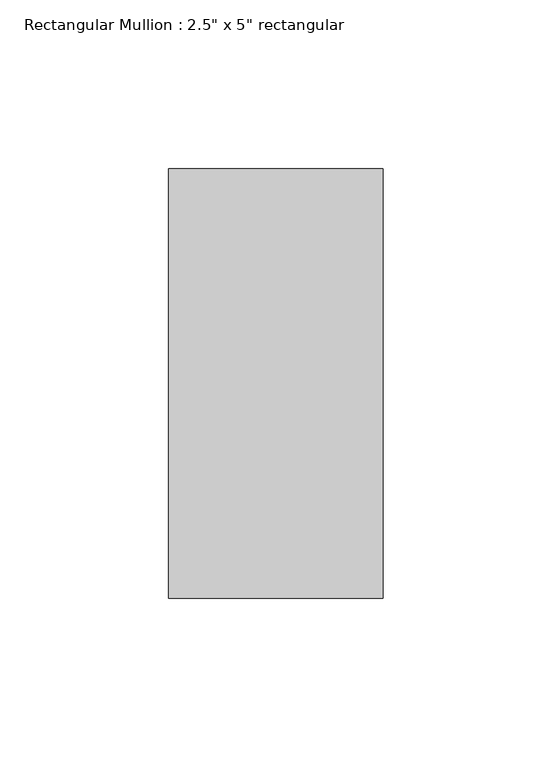
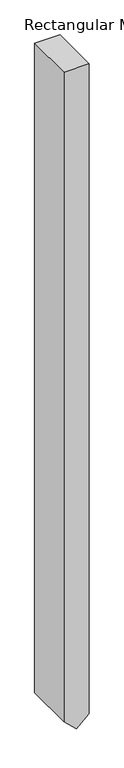
"""IFC4 building model written with IfcOpenShell, lengths in millimetres: member geometry."""

from ifc_helpers import new_model, si_unit, frame, origin, place, context, project, spatial, polyline, outline, extrude, source, transform, mapped, element, save


def member_2e3f679f(model_context):
    return source(origin(), model_context, "Body", "SweptSolid", [
        extrude(outline(polyline([(0.0, 31.75), (0.0, -31.75), (-1725.8468822, -31.75), (-1755.4542362, 0.0), (-1725.8468822, 31.75), (0.0, 31.75)])), frame((0.0, -63.5, 0.0), z_axis=(0.0, 1.0, 0.0), x_axis=(0.0, 0.0, 1.0)), (0.0, 0.0, 1.0), 127.0),
    ])


if __name__ == "__main__":
    model = new_model("IFC4")
    model_context = context("Model", 3, world=origin())
    ifc_project = project(units=[si_unit("LENGTHUNIT", "METRE", prefix="MILLI")], contexts=[model_context])
    site = spatial("IfcSite", under=ifc_project)
    building = spatial("IfcBuilding", under=site)
    placement = place(None, origin())
    member_shape = member_2e3f679f(model_context)
    element("IfcMember", 1, ObjectType="Rectangular Mullion : 2.5\" x 5\" rectangular", at=placement, inside=building, context=model_context, shape_type="MappedRepresentation", body=[
        mapped(member_shape, transform((0.0, 0.0, 0.0), x_axis=(1.0, 0.0, 0.0), y_axis=(0.0, 1.0, 0.0), z_axis=(0.0, 0.0, 1.0))),
    ])
    save(model, "model.ifc")

# Revit data of these elements
# Type "Rectangular Mullion : 2.5\" x 5\" rectangular"
#   built-in parameter 1007304 = 0.416667 (stored number, unit not read)
#   built-in parameter 1007301 = 0.104167 (stored number, unit not read)
#   built-in parameter 1007300 = 0.104167 (stored number, unit not read)
# Element 1 (IfcMember, "Rectangular Mullion : 2.5\" x 5\" rectangular")
#   Materials on its faces: "door colour"
# Materials
#   "door colour": class "Generic", colour RGB 120 120 120, transparency 0, Cost = 0
